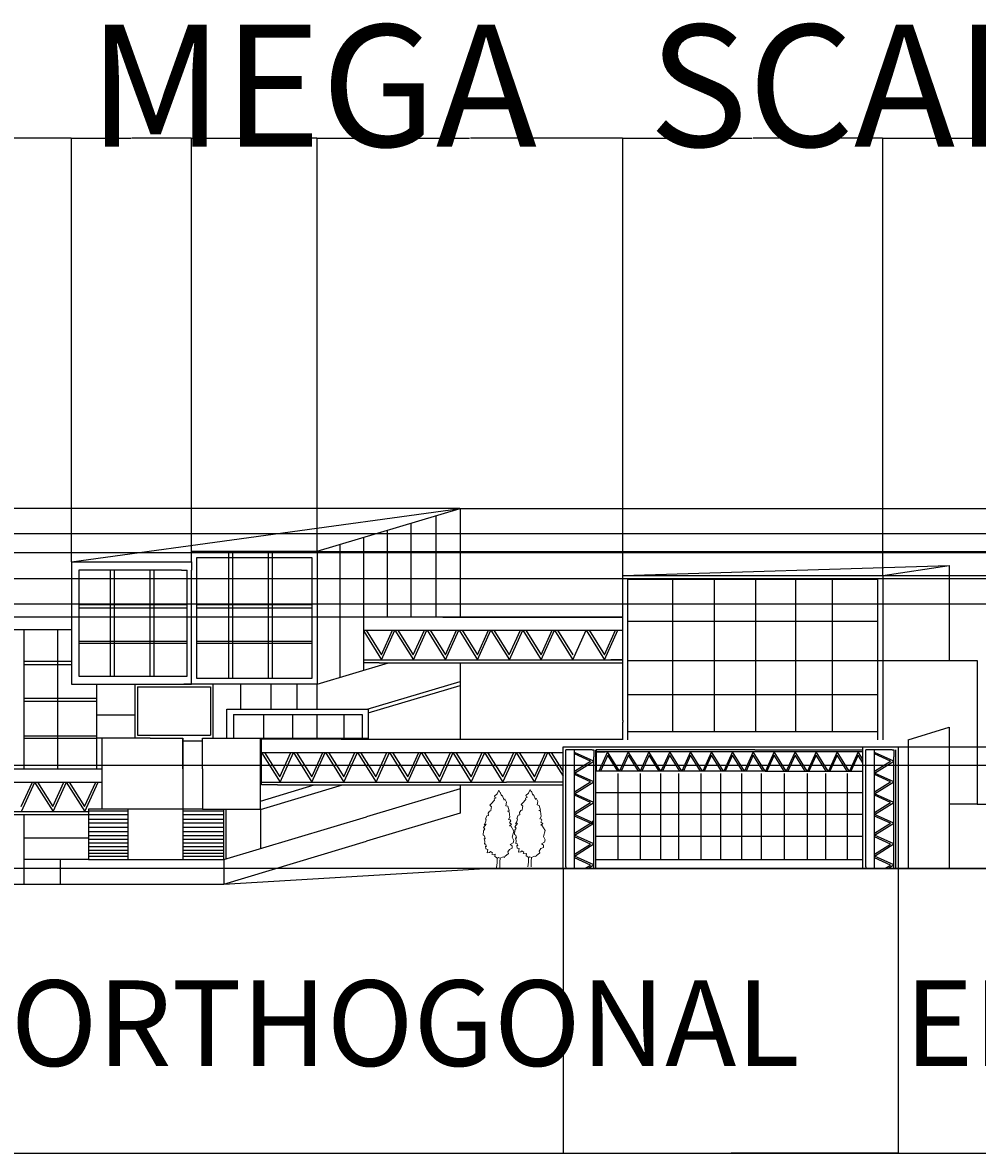
# Model space of a CAD drawing. Units: inches. Extents: x -2248 to 2617, y -128 to 922.
# Tile 2 of 7: x -1531 to -646, y -128 to 922. Entities that reach past the tile are written whole.
import ezdxf

# ---------------------------------------------------------------- set-up
doc = ezdxf.new("R2010")
doc.units = ezdxf.units.IN
doc.header["$MEASUREMENT"] = 0
for name, color, linetype, lineweight in [('A-ANNO-DIMS', 2, 'Continuous', 18), ('A-ANNO-TEXT', 7, 'Continuous', 25), ('A-ELEV', 7, 'Continuous', 25), ('L-PLNT', 3, 'Continuous', 18)]:
    doc.layers.add(name, color=color, linetype=linetype, lineweight=lineweight)
doc.styles.get("Standard").update_dxf_attribs({"font": 'arial.ttf'})
doc.dimstyles.get("Standard").update_dxf_attribs({"dimtxt": 0.18, "dimasz": 0.18, "dimexe": 0.18, "dimexo": 0.0625, "dimgap": 0.09, "dimtad": 0, "dimtih": 1, "dimtoh": 1, "dimdec": 4, "dimzin": 0, "dimdsep": 46, "dimtxsty": 'Standard', "dimcen": 0.09, "dimadec": 0, "dimazin": 0, "dimtfac": 1, "dimtdec": 4, "dimtofl": 0, "dimtmove": 0, "dimatfit": 3, "dimfxl": 1, "dimtolj": 1, "dimtzin": 0, "dimarcsym": 0})

# ---------------------------------------------------------------- blocks, each defined once
blk = doc.blocks.new('*U3')
blk.add_lwpolyline([(-2.754, 191.699), (-6.78, 182.851), (-13.682, 176.953), (-11.956, 173.266), (-9.656, 172.529), (-14.257, 170.317), (-13.682, 167.368), (-21.733, 157.783), (-25.184, 154.834), (-21.158, 150.41), (-21.733, 147.461), (-22.884, 140.825), (-26.334, 140.087), (-29.21, 134.926), (-28.635, 129.028), (-32.661, 128.291), (-36.111, 120.18), (-34.386, 118.706), (-35.536, 111.333), (-38.987, 106.171), (-34.386, 107.646), (-40.712, 98.798), (-37.261, 95.849), (-40.712, 90.688), (-41.287, 80.366), (-38.412, 78.154), (-36.686, 70.781), (-39.562, 71.518), (-37.261, 64.145), (-38.412, 57.509), (-36.111, 58.247), (-33.236, 52.348), (-35.536, 53.086), (-34.961, 46.45), (-30.36, 44.975), (-31.51, 36.128), (-26.334, 36.865), (-23.459, 39.814), (-18.283, 36.128), (-20.008, 33.178), (-14.832, 31.704), (-11.956, 33.178), (-12.531, 27.28), (-6.205, 22.856), (-3.905, 24.331), (0.121, 22.856), (8.173, 26.543), (11.624, 25.068), (12.199, 27.28), (21.4, 34.653), (19.675, 39.077), (23.701, 44.975), (30.027, 47.924), (30.602, 53.823), (25.426, 56.772), (32.903, 61.196), (34.053, 67.094), (30.602, 75.205), (34.628, 89.951), (26.576, 103.222), (23.701, 103.222), (28.302, 107.646), (23.701, 110.595), (26.576, 115.756), (25.426, 117.968), (20.825, 118.706), (24.276, 124.604), (22.551, 137.876), (19.1, 139.35), (22.551, 140.825), (19.675, 151.884), (14.499, 153.359), (16.224, 162.207), (12.199, 170.317), (10.473, 167.368), (5.872, 179.165), (4.147, 177.69), (0.696, 187.275), (-0.454, 185.8)], close=True)
for points in [[(-6.813, 23.669), (-6.813, 11.669), (-8.627, 0)], [(0.387, 23.669), (-0.576, 13.271), (-0.576, 3.686), (0, 0)]]:
    blk.add_lwpolyline(points)
blk = doc.blocks.new('*D19')
at = {"layer": 'A-ANNO-DIMS', "color": 0, "lineweight": -2, "transparency": 16777216}
for p, q in [((-1125.5, 470.6), (-2247.7, 470.6)), ((-2247.5, 470.4), (-2247.5, 438.4)), ((-2247.5, 406), (-2247.5, 438)), ((-1769.5, 405.8), (-2247.7, 405.8))]:
    blk.add_line(p, q, dxfattribs=at)
at = {"layer": 'A-ANNO-DIMS', "color": 0, "transparency": 16777216}
for points in [[(-2247.5, 470.4), (-2247.5, 470.4), (-2247.5, 470.6)], [(-2247.5, 406), (-2247.5, 406), (-2247.5, 405.8)]]:
    blk.add_solid(points, dxfattribs=at)
at = {"layer": 'Defpoints', "color": 0, "transparency": 16777216}
for p in [(-1125.4, 470.6), (-2247.5, 405.8), (-1769.4, 405.8)]:
    blk.add_point(p, dxfattribs=at)
at = {"layer": 'A-ANNO-DIMS', "color": 0, "transparency": 16777216, "insert": (-2247.5, 438.2), "char_height": 0.18, "attachment_point": 5}
blk.add_mtext('\\A1;64.83', dxfattribs=at)
blk = doc.blocks.new('*D20')
at = {"layer": 'A-ANNO-DIMS', "color": 0, "lineweight": -2, "transparency": 16777216}
for p, q in [((-1595.3, 429.9), (2616.5, 429.9)), ((2616.3, 429.7), (2616.3, 417.9)), ((2616.3, 405.8), (2616.3, 417.5)), ((-1653.9, 405.6), (2616.5, 405.6))]:
    blk.add_line(p, q, dxfattribs=at)
at = {"layer": 'A-ANNO-DIMS', "color": 0, "transparency": 16777216}
for points in [[(2616.2, 429.7), (2616.3, 429.7), (2616.3, 429.9)], [(2616.2, 405.8), (2616.3, 405.8), (2616.3, 405.6)]]:
    blk.add_solid(points, dxfattribs=at)
at = {"layer": 'Defpoints', "color": 0, "transparency": 16777216}
for p in [(-1595.4, 429.9), (-1654, 405.6), (2616.3, 405.6)]:
    blk.add_point(p, dxfattribs=at)
at = {"layer": 'A-ANNO-DIMS', "color": 0, "transparency": 16777216, "insert": (2616.3, 417.7), "char_height": 0.18, "attachment_point": 5}
blk.add_mtext('\\A1;24.3', dxfattribs=at)
blk = doc.blocks.new('*D21')
at = {"layer": 'A-ANNO-DIMS', "color": 0, "lineweight": -2, "transparency": 16777216}
for p, q in [((-1125.3, 470.6), (2616.5, 470.6)), ((2616.3, 470.4), (2616.3, 451)), ((2616.3, 431.1), (2616.3, 450.6)), ((-1257.9, 430.9), (2616.5, 430.9))]:
    blk.add_line(p, q, dxfattribs=at)
at = {"layer": 'A-ANNO-DIMS', "color": 0, "transparency": 16777216}
for points in [[(2616.2, 470.4), (2616.3, 470.4), (2616.3, 470.6)], [(2616.2, 431.1), (2616.3, 431.1), (2616.3, 430.9)]]:
    blk.add_solid(points, dxfattribs=at)
at = {"layer": 'Defpoints', "color": 0, "transparency": 16777216}
for p in [(-1125.4, 470.6), (-1258, 430.9), (2616.3, 430.9)]:
    blk.add_point(p, dxfattribs=at)
at = {"layer": 'A-ANNO-DIMS', "color": 0, "transparency": 16777216, "insert": (2616.3, 450.8), "char_height": 0.18, "attachment_point": 5}
blk.add_mtext('\\A1;39.705', dxfattribs=at)
blk = doc.blocks.new('*D22')
at = {"layer": 'A-ANNO-DIMS', "color": 0, "lineweight": -2, "transparency": 16777216}
for p, q in [((-733.3, 408.4), (2616.5, 408.4)), ((2616.3, 408.2), (2616.3, 329.1)), ((2616.3, 249.6), (2616.3, 328.7)), ((-719.1, 249.4), (2616.5, 249.4))]:
    blk.add_line(p, q, dxfattribs=at)
at = {"layer": 'A-ANNO-DIMS', "color": 0, "transparency": 16777216}
for points in [[(2616.2, 408.2), (2616.3, 408.2), (2616.3, 408.4)], [(2616.2, 249.6), (2616.3, 249.6), (2616.3, 249.4)]]:
    blk.add_solid(points, dxfattribs=at)
at = {"layer": 'Defpoints', "color": 0, "transparency": 16777216}
for p in [(-733.4, 408.4), (-719.2, 249.4), (2616.3, 249.4)]:
    blk.add_point(p, dxfattribs=at)
at = {"layer": 'A-ANNO-DIMS', "color": 0, "transparency": 16777216, "insert": (2616.3, 328.9), "char_height": 0.18, "attachment_point": 5}
blk.add_mtext('\\A1;159.02', dxfattribs=at)
blk = doc.blocks.new('*D23')
at = {"layer": 'A-ANNO-DIMS', "color": 0, "lineweight": -2, "transparency": 16777216}
for p, q in [((-719.1, 249.4), (2616.5, 249.4)), ((2616.3, 249.2), (2616.3, 193.1)), ((2616.3, 136.6), (2616.3, 192.7)), ((-719.1, 136.5), (2616.5, 136.5))]:
    blk.add_line(p, q, dxfattribs=at)
at = {"layer": 'A-ANNO-DIMS', "color": 0, "transparency": 16777216}
for points in [[(2616.2, 249.2), (2616.3, 249.2), (2616.3, 249.4)], [(2616.2, 136.6), (2616.3, 136.6), (2616.3, 136.5)]]:
    blk.add_solid(points, dxfattribs=at)
at = {"layer": 'Defpoints', "color": 0, "transparency": 16777216}
for p in [(-719.2, 249.4), (-719.2, 136.5), (2616.3, 136.5)]:
    blk.add_point(p, dxfattribs=at)
at = {"layer": 'A-ANNO-DIMS', "color": 0, "transparency": 16777216, "insert": (2616.3, 192.9), "char_height": 0.18, "attachment_point": 5}
blk.add_mtext('\\A1;112.94', dxfattribs=at)
blk = doc.blocks.new('*D29')
at = {"layer": 'A-ANNO-DIMS', "color": 0, "lineweight": -2, "transparency": 16777216}
for p, q in [((358.9, 382), (-2247.7, 382)), ((-2247.5, 381.8), (-2247.5, 259.4)), ((-2247.5, 136.6), (-2247.5, 259)), ((392.6, 136.5), (-2247.7, 136.5))]:
    blk.add_line(p, q, dxfattribs=at)
at = {"layer": 'A-ANNO-DIMS', "color": 0, "transparency": 16777216}
for points in [[(-2247.5, 381.8), (-2247.5, 381.8), (-2247.5, 382)], [(-2247.5, 136.6), (-2247.5, 136.6), (-2247.5, 136.5)]]:
    blk.add_solid(points, dxfattribs=at)
at = {"layer": 'Defpoints', "color": 0, "transparency": 16777216}
for p in [(359, 382), (-2247.5, 136.5), (392.7, 136.5)]:
    blk.add_point(p, dxfattribs=at)
at = {"layer": 'A-ANNO-DIMS', "color": 0, "transparency": 16777216, "insert": (-2247.5, 259.2), "char_height": 0.18, "attachment_point": 5}
blk.add_mtext('\\A1;245.5', dxfattribs=at)
blk = doc.blocks.new('*D30')
at = {"layer": 'A-ANNO-DIMS', "color": 0, "lineweight": -2, "transparency": 16777216}
for p, q in [((201.8, 232.1), (-2247.7, 232.1)), ((-2247.5, 231.9), (-2247.5, 184.4)), ((-2247.5, 136.6), (-2247.5, 184.1)), ((210.7, 136.5), (-2247.7, 136.5))]:
    blk.add_line(p, q, dxfattribs=at)
at = {"layer": 'A-ANNO-DIMS', "color": 0, "transparency": 16777216}
for points in [[(-2247.5, 231.9), (-2247.5, 231.9), (-2247.5, 232.1)], [(-2247.5, 136.6), (-2247.5, 136.6), (-2247.5, 136.5)]]:
    blk.add_solid(points, dxfattribs=at)
at = {"layer": 'Defpoints', "color": 0, "transparency": 16777216}
for p in [(201.8, 232.1), (-2247.5, 136.5), (210.8, 136.5)]:
    blk.add_point(p, dxfattribs=at)
at = {"layer": 'A-ANNO-DIMS', "color": 0, "transparency": 16777216, "insert": (-2247.5, 184.3), "char_height": 0.18, "attachment_point": 5}
blk.add_mtext('\\A1;95.6', dxfattribs=at)
blk = doc.blocks.new('*D31')
at = {"layer": 'A-ANNO-DIMS', "color": 0, "lineweight": -2, "transparency": 16777216}
for p, q in [((934.8, 447.2), (-2247.7, 447.2)), ((-2247.5, 447), (-2247.5, 292)), ((-2247.5, 136.6), (-2247.5, 291.6)), ((820, 136.5), (-2247.7, 136.5))]:
    blk.add_line(p, q, dxfattribs=at)
at = {"layer": 'A-ANNO-DIMS', "color": 0, "transparency": 16777216}
for points in [[(-2247.5, 447), (-2247.5, 447), (-2247.5, 447.2)], [(-2247.5, 136.6), (-2247.5, 136.6), (-2247.5, 136.5)]]:
    blk.add_solid(points, dxfattribs=at)
at = {"layer": 'Defpoints', "color": 0, "transparency": 16777216}
for p in [(934.9, 447.2), (-2247.5, 136.5), (820.1, 136.5)]:
    blk.add_point(p, dxfattribs=at)
at = {"layer": 'A-ANNO-DIMS', "color": 0, "transparency": 16777216, "insert": (-2247.5, 291.8), "char_height": 0.18, "attachment_point": 5}
blk.add_mtext('\\A1;310.7', dxfattribs=at)
blk = doc.blocks.new('*D32')
at = {"layer": 'A-ANNO-DIMS', "color": 0, "lineweight": -2, "transparency": 16777216}
for p, q in [((-975.3, 369.9), (-2247.7, 369.9)), ((-2247.5, 369.8), (-2247.5, 253.4)), ((-2247.5, 136.6), (-2247.5, 253)), ((-1029.9, 136.5), (-2247.7, 136.5))]:
    blk.add_line(p, q, dxfattribs=at)
at = {"layer": 'A-ANNO-DIMS', "color": 0, "transparency": 16777216}
for points in [[(-2247.5, 369.8), (-2247.5, 369.8), (-2247.5, 369.9)], [(-2247.5, 136.6), (-2247.5, 136.6), (-2247.5, 136.5)]]:
    blk.add_solid(points, dxfattribs=at)
at = {"layer": 'Defpoints', "color": 0, "transparency": 16777216}
for p in [(-975.2, 369.9), (-2247.5, 136.5), (-1029.8, 136.5)]:
    blk.add_point(p, dxfattribs=at)
at = {"layer": 'A-ANNO-DIMS', "color": 0, "transparency": 16777216, "insert": (-2247.5, 253.2), "char_height": 0.18, "attachment_point": 5}
blk.add_mtext('\\A1;233.5', dxfattribs=at)
blk = doc.blocks.new('*D33')
at = {"layer": 'A-ANNO-DIMS', "color": 0, "lineweight": -2, "transparency": 16777216}
for p, q in [((2393, 136.4), (2393, -127.9)), ((-2024.3, 122), (-2024.3, -127.9)), ((-2024.1, -127.7), (184, -127.7)), ((2392.8, -127.7), (184.7, -127.7))]:
    blk.add_line(p, q, dxfattribs=at)
at = {"layer": 'A-ANNO-DIMS', "color": 0, "transparency": 16777216}
for points in [[(-2024.1, -127.6), (-2024.1, -127.7), (-2024.3, -127.7)], [(2392.8, -127.6), (2392.8, -127.7), (2393, -127.7)]]:
    blk.add_solid(points, dxfattribs=at)
at = {"layer": 'Defpoints', "color": 0, "transparency": 16777216}
for p in [(2393, 136.5), (-2024.3, 122.1), (2393, -127.7)]:
    blk.add_point(p, dxfattribs=at)
at = {"layer": 'A-ANNO-DIMS', "color": 0, "transparency": 16777216, "insert": (184.4, -127.7), "char_height": 0.18, "attachment_point": 5}
blk.add_mtext('\\A1;4417', dxfattribs=at)
blk = doc.blocks.new('*D36')
at = {"layer": 'A-ANNO-DIMS', "color": 0, "lineweight": -2, "transparency": 16777216}
for p, q in [((-1654, 405.6), (-1654, 814.7)), ((-1653.8, 814.5), (-1570.3, 814.5)), ((-1486, 814.5), (-1569.4, 814.5)), ((-1485.8, 421.2), (-1485.8, 814.7))]:
    blk.add_line(p, q, dxfattribs=at)
at = {"layer": 'A-ANNO-DIMS', "color": 0, "transparency": 16777216}
for points in [[(-1653.8, 814.5), (-1653.8, 814.5), (-1654, 814.5)], [(-1486, 814.5), (-1486, 814.5), (-1485.8, 814.5)]]:
    blk.add_solid(points, dxfattribs=at)
at = {"layer": 'Defpoints', "color": 0, "transparency": 16777216}
for p in [(-1485.8, 814.5), (-1485.8, 421.2), (-1654, 405.6)]:
    blk.add_point(p, dxfattribs=at)
at = {"layer": 'A-ANNO-DIMS', "color": 0, "transparency": 16777216, "insert": (-1569.9, 814.5), "char_height": 0.18, "attachment_point": 5}
blk.add_mtext('\\A1;168.15', dxfattribs=at)
blk = doc.blocks.new('*D37')
at = {"layer": 'A-ANNO-DIMS', "color": 0, "lineweight": -2, "transparency": 16777216}
for p, q in [((-1485.8, 421.2), (-1485.8, 814.7)), ((-1485.6, 814.5), (-1430.6, 814.5)), ((-1374.8, 814.5), (-1429.8, 814.5)), ((-1374.6, 421.2), (-1374.6, 814.7))]:
    blk.add_line(p, q, dxfattribs=at)
at = {"layer": 'A-ANNO-DIMS', "color": 0, "transparency": 16777216}
for points in [[(-1485.6, 814.5), (-1485.6, 814.5), (-1485.8, 814.5)], [(-1374.8, 814.5), (-1374.8, 814.5), (-1374.6, 814.5)]]:
    blk.add_solid(points, dxfattribs=at)
at = {"layer": 'Defpoints', "color": 0, "transparency": 16777216}
for p in [(-1374.6, 814.5), (-1485.8, 421.2), (-1374.6, 421.2)]:
    blk.add_point(p, dxfattribs=at)
at = {"layer": 'A-ANNO-DIMS', "color": 0, "transparency": 16777216, "insert": (-1430.2, 814.5), "char_height": 0.18, "attachment_point": 5}
blk.add_mtext('\\A1;111.2', dxfattribs=at)
blk = doc.blocks.new('*D38')
at = {"layer": 'A-ANNO-DIMS', "color": 0, "lineweight": -2, "transparency": 16777216}
for p, q in [((-1374.6, 431), (-1374.6, 814.7)), ((-1374.4, 814.5), (-1316.7, 814.5)), ((-1258.1, 814.5), (-1315.8, 814.5)), ((-1258, 431), (-1258, 814.7))]:
    blk.add_line(p, q, dxfattribs=at)
at = {"layer": 'A-ANNO-DIMS', "color": 0, "transparency": 16777216}
for points in [[(-1374.4, 814.5), (-1374.4, 814.5), (-1374.6, 814.5)], [(-1258.1, 814.5), (-1258.1, 814.5), (-1258, 814.5)]]:
    blk.add_solid(points, dxfattribs=at)
at = {"layer": 'Defpoints', "color": 0, "transparency": 16777216}
for p in [(-1258, 814.5), (-1374.6, 430.9), (-1258, 430.9)]:
    blk.add_point(p, dxfattribs=at)
at = {"layer": 'A-ANNO-DIMS', "color": 0, "transparency": 16777216, "insert": (-1316.3, 814.5), "char_height": 0.18, "attachment_point": 5}
blk.add_mtext('\\A1;116.66', dxfattribs=at)
blk = doc.blocks.new('*D39')
at = {"layer": 'A-ANNO-DIMS', "color": 0, "lineweight": -2, "transparency": 16777216}
for p, q in [((-1258, 431), (-1258, 814.7)), ((-1257.8, 814.5), (-1116.7, 814.5)), ((-974.6, 814.5), (-1115.7, 814.5)), ((-974.4, 408.5), (-974.4, 814.7))]:
    blk.add_line(p, q, dxfattribs=at)
at = {"layer": 'A-ANNO-DIMS', "color": 0, "transparency": 16777216}
for points in [[(-1257.8, 814.5), (-1257.8, 814.5), (-1258, 814.5)], [(-974.6, 814.5), (-974.6, 814.5), (-974.4, 814.5)]]:
    blk.add_solid(points, dxfattribs=at)
at = {"layer": 'Defpoints', "color": 0, "transparency": 16777216}
for p in [(-974.4, 814.5), (-1258, 430.9), (-974.4, 408.4)]:
    blk.add_point(p, dxfattribs=at)
at = {"layer": 'A-ANNO-DIMS', "color": 0, "transparency": 16777216, "insert": (-1116.2, 814.5), "char_height": 0.18, "attachment_point": 5}
blk.add_mtext('\\A1;283.54', dxfattribs=at)
blk = doc.blocks.new('*D40')
at = {"layer": 'A-ANNO-DIMS', "color": 0, "lineweight": -2, "transparency": 16777216}
for p, q in [((-974.4, 408.5), (-974.4, 814.7)), ((-974.2, 814.5), (-854.4, 814.5)), ((-733.6, 814.5), (-853.4, 814.5)), ((-733.4, 408.5), (-733.4, 814.7))]:
    blk.add_line(p, q, dxfattribs=at)
at = {"layer": 'A-ANNO-DIMS', "color": 0, "transparency": 16777216}
for points in [[(-974.2, 814.5), (-974.2, 814.5), (-974.4, 814.5)], [(-733.6, 814.5), (-733.6, 814.5), (-733.4, 814.5)]]:
    blk.add_solid(points, dxfattribs=at)
at = {"layer": 'Defpoints', "color": 0, "transparency": 16777216}
for p in [(-733.4, 814.5), (-974.4, 408.4), (-733.4, 408.4)]:
    blk.add_point(p, dxfattribs=at)
at = {"layer": 'A-ANNO-DIMS', "color": 0, "transparency": 16777216, "insert": (-853.9, 814.5), "char_height": 0.18, "attachment_point": 5}
blk.add_mtext('\\A1;241.04', dxfattribs=at)
blk = doc.blocks.new('*D41')
at = {"layer": 'A-ANNO-DIMS', "color": 0, "lineweight": -2, "transparency": 16777216}
for p, q in [((-733.4, 408.5), (-733.4, 814.7)), ((-733.2, 814.5), (-649, 814.5)), ((-564.1, 814.5), (-648.2, 814.5)), ((-563.9, 327), (-563.9, 814.7))]:
    blk.add_line(p, q, dxfattribs=at)
at = {"layer": 'A-ANNO-DIMS', "color": 0, "transparency": 16777216}
for points in [[(-733.2, 814.5), (-733.2, 814.5), (-733.4, 814.5)], [(-564.1, 814.5), (-564.1, 814.5), (-563.9, 814.5)]]:
    blk.add_solid(points, dxfattribs=at)
at = {"layer": 'Defpoints', "color": 0, "transparency": 16777216}
for p in [(-563.9, 814.5), (-733.4, 408.4), (-563.9, 326.9)]:
    blk.add_point(p, dxfattribs=at)
at = {"layer": 'A-ANNO-DIMS', "color": 0, "transparency": 16777216, "insert": (-648.6, 814.5), "char_height": 0.18, "attachment_point": 5}
blk.add_mtext('\\A1;169.5', dxfattribs=at)
blk = doc.blocks.new('*D55')
at = {"layer": 'A-ANNO-DIMS', "color": 0, "lineweight": -2, "transparency": 16777216}
for p, q in [((-1029.8, 136.4), (-1029.8, -127.9)), ((-719.2, 136.4), (-719.2, -127.9)), ((-1029.6, -127.7), (-874.9, -127.7)), ((-719.4, -127.7), (-874.1, -127.7))]:
    blk.add_line(p, q, dxfattribs=at)
at = {"layer": 'A-ANNO-DIMS', "color": 0, "transparency": 16777216}
for points in [[(-1029.6, -127.6), (-1029.6, -127.7), (-1029.8, -127.7)], [(-719.4, -127.6), (-719.4, -127.7), (-719.2, -127.7)]]:
    blk.add_solid(points, dxfattribs=at)
at = {"layer": 'Defpoints', "color": 0, "transparency": 16777216}
for p in [(-1029.8, 136.5), (-719.2, 136.5), (-719.2, -127.7)]:
    blk.add_point(p, dxfattribs=at)
at = {"layer": 'A-ANNO-DIMS', "color": 0, "transparency": 16777216, "insert": (-874.5, -127.7), "char_height": 0.18, "attachment_point": 5}
blk.add_mtext('\\A1;310.6', dxfattribs=at)

msp = doc.modelspace()

# ---------------------------------------------------------------- linework, layer by layer
at = {"layer": 'A-ELEV'}
for p, q in [((-1485.8077, 421.1696), (-1125.4072, 470.6286)), ((-1257.9572, 430.9238), (-1125.4072, 470.6286)), ((-1147.628, 369.9469), (-1147.628, 463.9724)), ((-1125.4072, 470.6286), (-1125.4072, 369.9469)), ((-1170.7914, 369.9469), (-1170.7914, 457.0339)), ((-1214.6825, 320.7275), (-1214.6825, 443.8866)), ((-1192.7139, 369.9469), (-1192.7139, 450.4672)), ((-1374.6151, 421.1696), (-1374.6151, 430.9238)), ((-1374.6151, 430.9238), (-1257.9572, 430.9238)), ((-1339.8325, 312.9553), (-1339.8325, 430.9238)), ((-1336.0257, 312.9553), (-1336.0257, 430.9238)), ((-1303.0376, 312.9553), (-1303.0376, 430.9238)), ((-1299.2308, 312.9553), (-1299.2308, 430.9238)), ((-1257.9572, 430.9238), (-1257.9572, 307.4874)), ((-1236.5303, 314.1831), (-1236.5303, 437.3422)), ((-1485.8077, 421.1696), (-1485.8077, 307.4874)), ((-1485.8077, 421.1696), (-1381.4843, 421.1696)), ((-1381.4843, 421.1696), (-1374.6151, 421.1696)), ((-1374.6151, 421.1696), (-1374.6151, 413.422)), ((-1369.6504, 425.3485), (-1262.7839, 425.3485)), ((-1369.6504, 312.9553), (-1369.6504, 425.3485)), ((-1262.7839, 425.3485), (-1262.7839, 312.9553)), ((-1383.6311, 413.422), (-1478.9778, 413.422)), ((-1478.9778, 413.422), (-1478.9778, 315.1979)), ((-1449.7435, 315.1979), (-1449.7435, 413.422)), ((-1445.9367, 315.1979), (-1445.9367, 413.422)), ((-1412.9486, 315.1979), (-1412.9486, 413.422)), ((-1409.1418, 315.1979), (-1409.1418, 413.422)), ((-1383.6311, 413.422), (-1378.4219, 413.422)), ((-1378.4219, 315.1979), (-1378.4219, 413.422)), ((-1374.6151, 315.1979), (-1374.6151, 413.422)), ((-974.4198, 408.4102), (-671.7685, 417.6576)), ((-733.3752, 408.4102), (-671.7685, 417.6576)), ((-671.7685, 417.6576), (-671.7685, 329.7298)), ((-974.4198, 273.9094), (-974.4198, 408.4102)), ((-974.4198, 408.4102), (-733.3752, 408.4102)), ((-969.8646, 256.0775), (-969.8646, 405.203)), ((-969.8646, 405.203), (-738.371, 405.203)), ((-928.1701, 263.754), (-928.1701, 405.203)), ((-889.2644, 263.754), (-889.2644, 405.203)), ((-851.0598, 263.754), (-851.0598, 405.203)), ((-813.9067, 263.754), (-813.9067, 405.203)), ((-779.9081, 263.754), (-779.9081, 405.203)), ((-738.371, 405.203), (-738.371, 256.0775)), ((-733.3752, 408.4102), (-733.3752, 256.0775)), ((-1478.9778, 381.455), (-1378.4219, 381.455)), ((-1478.9778, 378.5661), (-1378.4219, 378.5661)), ((-1369.6504, 381.455), (-1262.7839, 381.455)), ((-1369.6504, 378.5661), (-1262.7839, 378.5661)), ((-1141.4884, 369.9469), (-1214.6825, 369.9469)), ((-1141.4884, 369.9469), (-975.2258, 369.9469)), ((-1595.3791, 358.31), (-1530.0359, 358.31)), ((-1530.0359, 358.31), (-1530.0359, 229.0275)), ((-1530.0359, 358.31), (-1485.8077, 358.31)), ((-1498.4948, 229.0275), (-1498.4948, 358.31)), ((-1214.6825, 357.7454), (-975.2258, 357.7454)), ((-1212.5193, 357.7367), (-1198.313, 334.9981)), ((-1198.313, 334.9981), (-1188.0363, 357.7454)), ((-1198.1833, 330.2906), (-1185.7808, 357.7433)), ((-1185.8244, 357.7454), (-1168.6715, 330.2906)), ((-1183.0075, 357.7367), (-1168.8011, 334.9981)), ((-1168.8011, 334.9981), (-1158.5244, 357.7454)), ((-1168.6715, 330.2906), (-1156.269, 357.7433)), ((-1156.0059, 357.7454), (-1138.853, 330.2906)), ((-1153.189, 357.7367), (-1138.9827, 334.9981)), ((-1138.9827, 334.9981), (-1128.7059, 357.7454)), ((-1138.853, 330.2906), (-1126.4505, 357.7433)), ((-1126.2751, 357.7454), (-1109.1222, 330.2906)), ((-1123.4582, 357.7367), (-1109.2519, 334.9981)), ((-1109.2519, 334.9981), (-1098.9752, 357.7454)), ((-1109.1222, 330.2906), (-1096.7197, 357.7433)), ((-1096.7476, 357.7454), (-1079.5947, 330.2906)), ((-1093.9307, 357.7367), (-1079.7243, 334.9981)), ((-1079.7243, 334.9981), (-1069.4476, 357.7454)), ((-1079.5947, 330.2906), (-1067.1922, 357.7433)), ((-1067.22, 357.7454), (-1050.0671, 330.2906)), ((-1064.4031, 357.7367), (-1050.1968, 334.9981)), ((-1050.1968, 334.9981), (-1039.9201, 357.7454)), ((-1050.0671, 330.2906), (-1037.6646, 357.7433)), ((-1037.918, 357.7454), (-1020.765, 330.2906)), ((-1035.101, 357.7367), (-1020.8947, 334.9981)), ((-1020.765, 330.2906), (-1008.3625, 357.7433)), ((-1008.5359, 357.7454), (-991.3829, 330.2906)), ((-1005.7189, 357.7367), (-991.5126, 334.9981)), ((-991.5126, 334.9981), (-981.2359, 357.7454)), ((-991.3829, 330.2906), (-978.9804, 357.7433)), ((-969.8646, 365.9872), (-738.371, 365.9872)), ((-1478.9778, 347.6299), (-1378.4219, 347.6299)), ((-1369.6504, 347.6299), (-1262.7839, 347.6299)), ((-1214.6825, 356.6991), (-1198.1833, 330.2906)), ((-1478.9778, 345.6601), (-1378.4219, 345.6601)), ((-1369.6504, 345.6601), (-1262.7839, 345.6601)), ((-1530.0359, 328.9999), (-1485.8077, 328.9999)), ((-1530.0359, 325.9078), (-1485.8077, 325.9078)), ((-1257.9572, 307.7647), (-1191.8127, 327.578)), ((-1214.6825, 330.2635), (-974.4198, 330.2635)), ((-1200.437, 327.578), (-1214.6825, 327.578)), ((-1200.437, 327.578), (-974.4198, 327.578)), ((-1125.4072, 327.578), (-1125.4072, 256.4375)), ((-987.9902, 327.578), (-975.2258, 327.578)), ((-975.2258, 330.2635), (-985.4566, 330.2635)), ((-969.8646, 329.7298), (-738.371, 329.7298)), ((-738.371, 329.7298), (-645.8648, 329.7298)), ((-645.8648, 329.7298), (-645.8648, 196.2696)), ((-1478.9778, 315.1979), (-1381.4843, 315.1979)), ((-1381.4843, 315.1979), (-1378.4219, 315.1979)), ((-1374.6151, 307.4874), (-1374.6151, 315.1979)), ((-1485.8077, 307.4874), (-1381.4843, 307.4874)), ((-1462.7609, 307.4874), (-1462.7609, 229.0275)), ((-1426.9499, 307.4874), (-1426.9499, 257.552)), ((-1424.4443, 305.1388), (-1424.4443, 260.2412)), ((-1424.4443, 305.1388), (-1356.8422, 305.1388)), ((-1381.4843, 307.4874), (-1374.6151, 307.4874)), ((-1257.9572, 307.4874), (-1381.4843, 307.4874)), ((-1262.7839, 312.9553), (-1369.6504, 312.9553)), ((-1356.8422, 305.1388), (-1356.8422, 260.2412)), ((-1354.5526, 257.552), (-1354.5526, 307.4874)), ((-1328.7904, 284.3577), (-1328.7904, 307.4874)), ((-1300.4636, 284.3577), (-1300.4636, 307.4874)), ((-1276.6333, 284.3577), (-1276.6333, 307.4874)), ((-1257.9572, 284.3577), (-1257.9572, 307.4874)), ((-1211.7192, 284.3577), (-1125.4072, 310.2121)), ((-1210.5891, 280.9745), (-1125.4072, 306.4903)), ((-1530.0359, 294.6973), (-1462.7609, 294.6973)), ((-974.4198, 273.9094), (-974.4198, 298.3514)), ((-969.8646, 298.1516), (-738.371, 298.1516)), ((-1530.0359, 291.9114), (-1462.7609, 291.9114)), ((-1341.6517, 257.552), (-1341.6517, 284.3577)), ((-1341.6517, 284.3577), (-1210.5891, 284.3577)), ((-1210.5891, 284.3577), (-1210.5891, 256.4375)), ((-1462.7609, 279.1363), (-1426.9499, 279.1363)), ((-1335.6667, 279.3427), (-1216.2013, 279.3427)), ((-1335.6667, 279.3427), (-1335.6667, 257.552)), ((-1307.2842, 257.552), (-1307.2842, 279.3427)), ((-1280.4676, 257.552), (-1280.4676, 279.3427)), ((-1257.9927, 257.552), (-1257.9927, 279.3427)), ((-1232.9967, 257.552), (-1232.9967, 279.3427)), ((-1216.2013, 279.3427), (-1216.2013, 257.552)), ((-974.4198, 273.9094), (-974.4198, 272.4308)), ((-974.4198, 256.0775), (-974.4198, 272.4308)), ((-969.8646, 263.754), (-738.371, 263.754)), ((-709.8168, 256.0775), (-671.7685, 267.5832)), ((-671.7685, 267.5832), (-671.7685, 196.2696)), ((-1530.0359, 259.7188), (-1462.7609, 259.7188)), ((-1530.0359, 257.552), (-1462.7609, 257.552)), ((-1412.9486, 257.552), (-1462.7609, 257.552)), ((-1457.3701, 229.0275), (-1457.3701, 257.552)), ((-1424.4443, 260.2412), (-1356.8422, 260.2412)), ((-1412.9486, 257.552), (-1382.6193, 257.552)), ((-1382.6193, 229.0275), (-1382.6193, 257.552)), ((-1382.6193, 257.552), (-1382.6193, 191.6077)), ((-1382.6193, 255.0357), (-1364.4124, 255.0357)), ((-1364.4124, 229.0275), (-1364.4124, 257.552)), ((-1364.4124, 257.552), (-1257.9572, 257.552)), ((-1310.5836, 229.0275), (-1310.5836, 257.552)), ((-1235.7073, 256.4375), (-1310.5836, 256.4375)), ((-1309.5551, 216.754), (-1309.5551, 256.4375)), ((-1257.9927, 257.552), (-1210.5891, 257.552)), ((-1257.9572, 257.552), (-1257.9572, 257.7708)), ((-1235.7073, 256.4375), (-974.4198, 256.4375)), ((-709.8168, 256.0775), (-709.8168, 136.4519)), ((-1309.5551, 244.236), (-1029.8099, 244.236)), ((-1309.5551, 244.236), (-1292.4022, 216.7812)), ((-1306.7382, 244.2273), (-1292.5319, 221.4887)), ((-1292.5319, 221.4887), (-1282.2552, 244.236)), ((-1292.4022, 216.7812), (-1279.9997, 244.2338)), ((-1280.0433, 244.236), (-1262.8904, 216.7812)), ((-1277.2264, 244.2273), (-1263.02, 221.4887)), ((-1263.02, 221.4887), (-1252.7433, 244.236)), ((-1262.8904, 216.7812), (-1250.4879, 244.2338)), ((-1250.2248, 244.236), (-1233.0719, 216.7812)), ((-1247.4079, 244.2273), (-1233.2016, 221.4887)), ((-1233.2016, 221.4887), (-1222.9248, 244.236)), ((-1233.0719, 216.7812), (-1220.6694, 244.2338)), ((-1220.494, 244.236), (-1203.3411, 216.7812)), ((-1217.6771, 244.2273), (-1203.4708, 221.4887)), ((-1203.4708, 221.4887), (-1193.1941, 244.236)), ((-1203.3411, 216.7812), (-1190.9386, 244.2338)), ((-1190.9665, 244.236), (-1173.8136, 216.7812)), ((-1188.1496, 244.2273), (-1173.9432, 221.4887)), ((-1173.9432, 221.4887), (-1163.6665, 244.236)), ((-1173.8136, 216.7812), (-1161.4111, 244.2338)), ((-1161.4389, 244.236), (-1144.286, 216.7812)), ((-1158.622, 244.2273), (-1144.4157, 221.4887)), ((-1144.4157, 221.4887), (-1134.139, 244.236)), ((-1144.286, 216.7812), (-1131.8835, 244.2338)), ((-1133.5882, 244.236), (-1134.2252, 244.0452)), ((-1133.5882, 244.236), (-1134.2252, 244.0452)), ((-1132.1369, 244.236), (-1114.9839, 216.7812)), ((-1129.3199, 244.2273), (-1115.1136, 221.4887)), ((-1115.1136, 221.4887), (-1104.8369, 244.236)), ((-1114.9839, 216.7812), (-1102.5814, 244.2338)), ((-1102.7548, 244.236), (-1085.6018, 216.7812)), ((-1099.9378, 244.2273), (-1085.7315, 221.4887)), ((-1085.7315, 221.4887), (-1075.4548, 244.236)), ((-1085.6018, 216.7812), (-1073.1993, 244.2338)), ((-1073.4557, 244.236), (-1056.3028, 216.7812)), ((-1070.6388, 244.2273), (-1056.4324, 221.4887)), ((-1056.4324, 221.4887), (-1046.1557, 244.236)), ((-1056.3028, 216.7812), (-1043.9003, 244.2338)), ((-1043.6169, 244.236), (-1029.8099, 222.1366)), ((-1040.8, 244.2273), (-1029.8099, 226.6366)), ((-1029.8099, 136.4519), (-1029.8099, 249.389)), ((-1029.8099, 249.389), (-719.1936, 249.389)), ((-1027.1698, 138.162), (-1027.1698, 246.762)), ((-1002.7278, 246.762), (-1027.1698, 246.762)), ((-1027.1698, 243.2408), (-1027.1698, 246.762)), ((-1019.2, 136.4519), (-1019.2, 246.762)), ((-1004.3419, 236.1238), (-1019.2, 242.8364)), ((-1001.267, 236.2085), (-1019.1986, 244.3096)), ((-1002.7278, 246.762), (-1001.2492, 246.762)), ((-1001.2492, 246.762), (-1001.2492, 240.0794)), ((-999.4951, 238.4246), (-999.4951, 246.762)), ((-990.7946, 246.7131), (-999.132, 246.7131)), ((-999.132, 246.7131), (-999.132, 243.4805)), ((-990.7946, 244.959), (-999.132, 244.959)), ((-999.132, 244.959), (-990.7946, 244.959)), ((-999.132, 243.4805), (-999.132, 227.0082)), ((-988.5785, 244.9413), (-996.6796, 227.0096)), ((-988.4938, 241.8664), (-995.2064, 227.0082)), ((-979.046, 246.7131), (-990.7946, 246.7131)), ((-751.6796, 244.959), (-990.7946, 244.959)), ((-977.3745, 227.0082), (-988.5785, 244.9413)), ((-979.2144, 227.0139), (-988.4938, 241.8664)), ((-852.0278, 246.7131), (-979.046, 246.7131)), ((-969.3866, 244.9413), (-977.4877, 227.0096)), ((-969.3019, 241.8664), (-976.0145, 227.0082)), ((-958.1826, 227.0082), (-969.3866, 244.9413)), ((-960.0225, 227.0139), (-969.3019, 241.8664)), ((-950.2469, 244.9413), (-958.348, 227.0096)), ((-950.1622, 241.8664), (-956.8748, 227.0082)), ((-939.0429, 227.0082), (-950.2469, 244.9413)), ((-940.8829, 227.0139), (-950.1622, 241.8664)), ((-947.8324, 244.9917), (-947.8503, 244.959)), ((-947.8174, 244.959), (-947.8324, 244.9917)), ((-930.96, 244.9413), (-939.0611, 227.0096)), ((-930.8753, 241.8664), (-937.5879, 227.0082)), ((-919.756, 227.0082), (-930.96, 244.9413)), ((-921.596, 227.0139), (-930.8753, 241.8664)), ((-911.6731, 244.9413), (-919.7742, 227.0096)), ((-911.5884, 241.8664), (-918.301, 227.0082)), ((-900.4691, 227.0082), (-911.6731, 244.9413)), ((-902.3091, 227.0139), (-911.5884, 241.8664)), ((-892.2534, 244.9413), (-900.3546, 227.0096)), ((-892.1687, 241.8664), (-898.8813, 227.0082)), ((-881.0494, 227.0082), (-892.2534, 244.9413)), ((-882.8894, 227.0139), (-892.1687, 241.8664)), ((-872.7765, 244.9413), (-880.8776, 227.0096)), ((-872.6918, 241.8664), (-879.4044, 227.0082)), ((-861.5725, 227.0082), (-872.7765, 244.9413)), ((-863.4125, 227.0139), (-872.6918, 241.8664)), ((-853.4998, 244.9413), (-861.601, 227.0096)), ((-853.4152, 241.8664), (-860.1277, 227.0082)), ((-842.2958, 227.0082), (-853.4998, 244.9413)), ((-844.1358, 227.0139), (-853.4152, 241.8664)), ((-852.0278, 246.5867), (-751.6796, 246.5867)), ((-834.1517, 244.9413), (-842.2528, 227.0096)), ((-834.067, 241.8664), (-840.7796, 227.0082)), ((-822.9477, 227.0082), (-834.1517, 244.9413)), ((-824.7877, 227.0139), (-834.067, 241.8664)), ((-814.7058, 244.9413), (-822.8069, 227.0096)), ((-814.6211, 241.8664), (-821.3337, 227.0082)), ((-803.5018, 227.0082), (-814.7058, 244.9413)), ((-805.3418, 227.0139), (-814.6211, 241.8664)), ((-795.2038, 244.9413), (-803.3049, 227.0096)), ((-795.1191, 241.8664), (-801.8317, 227.0082)), ((-783.9998, 227.0082), (-795.2038, 244.9413)), ((-785.8398, 227.0139), (-795.1191, 241.8664)), ((-775.6602, 244.9413), (-783.7613, 227.0096)), ((-775.5755, 241.8664), (-782.2881, 227.0082)), ((-764.4562, 227.0082), (-775.6602, 244.9413)), ((-766.2962, 227.0139), (-775.5755, 241.8664)), ((-756.2144, 244.9413), (-764.3155, 227.0096)), ((-756.1297, 241.8664), (-762.8423, 227.0082)), ((-751.6796, 237.683), (-756.2144, 244.9413)), ((-751.6796, 234.7437), (-756.1297, 241.8664)), ((-751.6796, 136.4519), (-751.6796, 249.389)), ((-749.0396, 138.162), (-749.0396, 246.762)), ((-724.5975, 246.762), (-749.0396, 246.762)), ((-749.0396, 243.2408), (-749.0396, 246.762)), ((-741.0698, 136.4519), (-741.0698, 246.762)), ((-726.2116, 236.1238), (-741.0698, 242.8364)), ((-723.1367, 236.2085), (-741.0684, 244.3096)), ((-724.5975, 246.762), (-723.119, 246.762)), ((-723.119, 246.762), (-723.119, 240.0794)), ((-721.3649, 238.4246), (-721.3649, 246.762)), ((-719.1936, 249.389), (-719.1936, 136.4519)), ((-1019.2, 225.0045), (-1001.267, 236.2085)), ((-1019.1943, 226.8444), (-1004.3419, 236.1238)), ((-1001.2492, 238.4246), (-1001.2492, 240.0794)), ((-1001.2492, 136.4519), (-1001.2492, 238.4246)), ((-999.4951, 226.676), (-999.4951, 238.4246)), ((-906.9389, 236.9224), (-906.9389, 236.9421)), ((-741.0698, 225.0045), (-723.1367, 236.2085)), ((-741.0641, 226.8444), (-726.2116, 236.1238)), ((-723.119, 238.4246), (-723.119, 240.0794)), ((-723.119, 136.4519), (-723.119, 238.4246)), ((-721.3649, 226.676), (-721.3649, 238.4246)), ((-1623.6327, 229.0275), (-1457.3701, 229.0275)), ((-1462.7609, 229.0275), (-1457.3701, 229.0275)), ((-1457.3701, 191.6077), (-1457.3701, 229.0275)), ((-1364.4124, 229.0275), (-1364.4124, 191.6077)), ((-1310.5836, 191.6077), (-1310.5836, 229.0275)), ((-1210.5891, 229.0578), (-1210.5891, 229.0275)), ((-1004.3419, 216.9319), (-1019.2, 223.6444)), ((-1001.267, 217.0165), (-1019.1986, 225.1177)), ((-999.4951, 136.4519), (-999.4951, 226.676)), ((-842.2958, 227.0082), (-999.132, 227.0082)), ((-979.2144, 224.7717), (-979.2144, 144.9711)), ((-958.4489, 224.7717), (-958.4489, 144.9711)), ((-957.2346, 227.0082), (-956.8185, 227.1329)), ((-957.2346, 227.0082), (-956.8185, 227.1329)), ((-939.6302, 224.7717), (-939.6302, 144.9711)), ((-922.7582, 224.7717), (-922.7582, 144.9711)), ((-901.9927, 224.7717), (-901.9927, 144.9711)), ((-883.8228, 224.7717), (-883.8228, 144.9711)), ((-864.3552, 224.7717), (-864.3552, 144.9711)), ((-846.1853, 224.7717), (-846.1853, 144.9711)), ((-842.2958, 227.0082), (-751.6796, 227.0082)), ((-824.7709, 224.7717), (-824.7709, 144.9711)), ((-803.3564, 224.7717), (-803.3564, 144.9711)), ((-786.4845, 224.7717), (-786.4845, 144.9711)), ((-766.3679, 224.7717), (-766.3679, 144.9711)), ((-726.2116, 216.9319), (-741.0698, 223.6444)), ((-723.1367, 217.0165), (-741.0684, 225.1177)), ((-721.3649, 136.4519), (-721.3649, 226.676)), ((-1697.4805, 216.8261), (-1457.3701, 216.8261)), ((-1532.341, 194.0788), (-1522.0643, 216.8261)), ((-1532.2114, 189.3712), (-1519.8089, 216.8239)), ((-1520.0622, 216.8261), (-1502.9093, 189.3712)), ((-1517.2453, 216.8173), (-1503.0389, 194.0788)), ((-1503.0389, 194.0788), (-1492.7622, 216.8261)), ((-1502.9093, 189.3712), (-1490.5068, 216.8239)), ((-1490.6801, 216.8261), (-1473.5272, 189.3712)), ((-1487.8632, 216.8173), (-1473.6568, 194.0788)), ((-1473.6568, 194.0788), (-1463.3801, 216.8261)), ((-1473.5272, 189.3712), (-1461.1247, 216.8239)), ((-1310.5836, 191.2179), (-1234.2989, 214.0685)), ((-1310.5836, 191.2179), (-1234.2989, 214.0685)), ((-1310.5836, 199.1049), (-1260.6289, 214.0685)), ((-1309.5551, 216.754), (-1082.2091, 216.754)), ((-1309.5551, 214.262), (-1309.5551, 216.754)), ((-1294.6559, 214.262), (-1309.5551, 214.262)), ((-1294.6559, 214.0685), (-1100.1957, 214.0685)), ((-1125.4072, 210.4985), (-1212.0466, 184.5461)), ((-1148.0055, 216.754), (-1147.9826, 216.704)), ((-1147.9826, 216.704), (-1147.9552, 216.754)), ((-1125.4072, 214.0685), (-1125.4072, 210.4985)), ((-1125.4072, 210.4985), (-1125.4072, 187.8086)), ((-1100.1957, 214.0685), (-1082.2091, 214.0685)), ((-1029.8099, 216.754), (-1082.2091, 216.754)), ((-1082.2091, 214.0685), (-1029.8099, 214.0685)), ((-1019.2, 205.8125), (-1001.267, 217.0165)), ((-1019.1943, 207.6525), (-1004.3419, 216.9319)), ((-741.0698, 205.8125), (-723.1367, 217.0165)), ((-741.0641, 207.6525), (-726.2116, 216.9319)), ((-1004.3419, 197.7922), (-1019.2, 204.5048)), ((-1001.267, 197.8769), (-1019.1986, 205.978)), ((-999.4951, 207.0277), (-751.6796, 207.0277)), ((-726.2116, 197.7922), (-741.0698, 204.5048)), ((-723.1367, 197.8769), (-741.0684, 205.978)), ((-1697.4805, 189.3441), (-1470.1344, 189.3441)), ((-1457.3701, 191.6077), (-1470.1344, 191.6077)), ((-1470.1344, 191.6077), (-1470.1344, 144.8414)), ((-1470.1344, 189.9991), (-1433.1251, 189.9991)), ((-1382.6193, 191.6077), (-1457.3701, 191.6077)), ((-1433.1251, 144.8414), (-1433.1251, 191.6077)), ((-1364.4124, 191.6077), (-1382.6193, 191.6077)), ((-1382.6193, 191.6077), (-1382.6193, 144.8414)), ((-1382.6193, 189.9991), (-1344.5966, 189.9991)), ((-1364.4124, 191.6077), (-1310.5836, 191.6077)), ((-1344.5966, 144.8414), (-1344.5966, 191.6077)), ((-1342.2527, 145.5435), (-1342.2527, 191.6077)), ((-1310.5836, 191.6077), (-1310.5836, 155.0298)), ((-1019.2, 186.6729), (-1001.267, 197.8769)), ((-1019.1943, 188.5129), (-1004.3419, 197.7922)), ((-1001.2166, 195.4623), (-1001.2492, 195.4802)), ((-1001.2492, 195.4474), (-1001.2166, 195.4623)), ((-741.0698, 186.6729), (-723.1367, 197.8769)), ((-741.0641, 188.5129), (-726.2116, 197.7922)), ((-723.0863, 195.4623), (-723.119, 195.4802)), ((-723.119, 195.4474), (-723.0863, 195.4623)), ((-645.8648, 196.2696), (-671.7685, 196.2696)), ((-671.7685, 196.2696), (-671.7685, 136.4519)), ((-645.8648, 196.2696), (-629.7186, 196.2696)), ((-1682.5813, 186.6586), (-1488.121, 186.6586)), ((-1530.0359, 186.6586), (-1530.0359, 122.0847)), ((-1488.121, 186.6586), (-1470.1344, 186.6586)), ((-1470.1344, 186.6586), (-1433.1251, 186.6586)), ((-1470.1344, 182.4099), (-1433.1251, 182.4099)), ((-1470.1344, 178.786), (-1433.1251, 178.786)), ((-1382.6193, 186.6586), (-1344.5966, 186.6586)), ((-1382.6193, 182.4099), (-1344.5966, 182.4099)), ((-1382.6193, 178.786), (-1344.5966, 178.786)), ((-1344.5966, 144.8414), (-1212.0466, 184.5461)), ((-1125.4072, 187.8086), (-1212.0466, 161.8562)), ((-1004.3419, 178.5053), (-1019.2, 185.2179)), ((-1019.2, 167.386), (-1001.267, 178.59)), ((-1001.267, 178.59), (-1019.1986, 186.6911)), ((-1019.1943, 169.2259), (-1004.3419, 178.5053)), ((-1004.3971, 178.5303), (-1002.3355, 178.5303)), ((-1002.3355, 177.9224), (-1002.3355, 180.7938)), ((-999.4951, 187.0261), (-751.6796, 187.0261)), ((-726.2116, 178.5053), (-741.0698, 185.2179)), ((-741.0698, 167.386), (-723.1367, 178.59)), ((-723.1367, 178.59), (-741.0684, 186.6911)), ((-741.0641, 169.2259), (-726.2116, 178.5053)), ((-1470.1344, 174.7872), (-1433.1251, 174.7872)), ((-1470.1344, 170.7884), (-1433.1251, 170.7884)), ((-1382.6193, 174.7872), (-1344.5966, 174.7872)), ((-1382.6193, 170.7884), (-1344.5966, 170.7884)), ((-1470.1344, 164.8394), (-1530.0359, 164.8394)), ((-1470.1344, 167.1645), (-1433.1251, 167.1645)), ((-1470.1344, 163.8757), (-1433.1251, 163.8757)), ((-1470.1344, 160.3768), (-1433.1251, 160.3768)), ((-1382.6193, 167.1645), (-1344.5966, 167.1645)), ((-1382.6193, 163.8757), (-1344.5966, 163.8757)), ((-1382.6193, 160.3768), (-1344.5966, 160.3768)), ((-1344.5966, 122.1515), (-1212.0466, 161.8562)), ((-1004.3419, 159.2184), (-1019.2, 165.931)), ((-1019.2, 148.0991), (-1001.267, 159.3031)), ((-1001.267, 159.3031), (-1019.1986, 167.4042)), ((-1019.1943, 149.939), (-1004.3419, 159.2184)), ((-999.4951, 166.4192), (-751.6796, 166.4192)), ((-726.2116, 159.2184), (-741.0698, 165.931)), ((-741.0698, 148.0991), (-723.1367, 159.3031)), ((-723.1367, 159.3031), (-741.0684, 167.4042)), ((-741.0641, 149.939), (-726.2116, 159.2184)), ((-1470.1344, 157.0028), (-1433.1251, 157.0028)), ((-1470.1344, 153.6288), (-1433.1251, 153.6288)), ((-1470.1344, 150.6297), (-1433.1251, 150.6297)), ((-1470.1344, 147.8805), (-1433.1251, 147.8805)), ((-1382.6193, 157.0028), (-1344.5966, 157.0028)), ((-1382.6193, 153.6288), (-1344.5966, 153.6288)), ((-1382.6193, 150.6297), (-1344.5966, 150.6297)), ((-1382.6193, 147.8805), (-1344.5966, 147.8805)), ((-1001.267, 139.8834), (-1019.1986, 147.9845)), ((-723.1367, 139.8834), (-741.0684, 147.9845)), ((-1496.3734, 144.8414), (-1530.0359, 144.8414)), ((-1470.1344, 144.8414), (-1496.3734, 144.8414)), ((-1496.3734, 144.8414), (-1496.3734, 122.0847)), ((-1470.1344, 144.8414), (-1441.1215, 144.8414)), ((-1441.1215, 144.8414), (-1344.5966, 144.8414)), ((-1344.5966, 144.8414), (-1344.5966, 122.0847)), ((-1344.5966, 122.0847), (-1102.1412, 136.4519)), ((-1102.1412, 136.4519), (-602.3282, 136.4519)), ((-1027.1698, 138.162), (-1027.1698, 136.4519)), ((-1004.3419, 139.7987), (-1019.2, 146.5113)), ((-1009.6988, 136.4519), (-1004.3419, 139.7987)), ((-1006.7595, 136.4519), (-1001.267, 139.8834)), ((-999.4951, 144.9711), (-751.6796, 144.9711)), ((-749.0396, 138.162), (-749.0396, 136.4519)), ((-726.2116, 139.7987), (-741.0698, 146.5113)), ((-731.5686, 136.4519), (-726.2116, 139.7987)), ((-728.6293, 136.4519), (-723.1367, 139.8834)), ((-1717.4681, 122.0847), (-1344.5966, 122.0847))]:
    msp.add_line(p, q, dxfattribs=at)

# ---------------------------------------------------------------- block references
at = {"layer": 'L-PLNT', "xscale": 0.373818396241174, "yscale": 0.373818396241174, "zscale": 0.373818396241174}
for p in [(-1088.4001, 137.5205), (-1059.3419, 138.1655)]:
    msp.add_blockref('*U3', p, dxfattribs=at)

# ---------------------------------------------------------------- texts
at = {"layer": 'A-ANNO-TEXT'}
for s, height, p in [('MEGA   SCALE   INSTITUTIONAL   COMPLEX    ', 113.064343, (-1470.2311, 806.5595)), ('FRONTH   ORTHOGONAL    ELEVATION', 79.456618, (-2046.3376, -46.7341))]:
    msp.add_text(s, height=height, dxfattribs=at).set_placement(p)

# ---------------------------------------------------------------- dimensions: what is measured, and where the dimension line sits
at = {"layer": 'A-ANNO-DIMS'}
for base, p1, p2, override, picture, middle in [((-1485.8077, 814.5189), (-1653.9599, 405.5754), (-1485.8077, 421.1696), {"dimdec": 2, "dimlfac": 1, "dimrnd": 0, "dimzin": 0, "dimdsep": 46, "dimlunit": 2}, '*D36', (-1569.8838, 814.5189)), ((-1374.6151, 814.5189), (-1485.8077, 421.1696), (-1374.6151, 421.1696), {"dimdec": 1, "dimlfac": 1, "dimrnd": 0, "dimzin": 0, "dimdsep": 46, "dimlunit": 2}, '*D37', (-1430.2114, 814.5189)), ((-1257.9572, 814.5189), (-1374.6151, 430.9238), (-1257.9572, 430.9238), {"dimdec": 2, "dimlfac": 1, "dimrnd": 0, "dimzin": 0, "dimdsep": 46, "dimlunit": 2}, '*D38', (-1316.2861, 814.5189)), ((-974.4198, 814.5189), (-1257.9572, 430.9238), (-974.4198, 408.4102), {"dimdec": 2, "dimlfac": 1, "dimrnd": 0, "dimzin": 0, "dimdsep": 46, "dimlunit": 2}, '*D39', (-1116.1885, 814.5189)), ((-733.3752, 814.5189), (-974.4198, 408.4102), (-733.3752, 408.4102), {"dimdec": 2, "dimlfac": 1, "dimrnd": 0, "dimzin": 0, "dimdsep": 46, "dimlunit": 2}, '*D40', (-853.8975, 814.5189)), ((-563.8805, 814.5189), (-733.3752, 408.4102), (-563.8805, 326.8999), {"dimdec": 1, "dimlfac": 1, "dimrnd": 0, "dimzin": 0, "dimdsep": 46, "dimlunit": 2}, '*D41', (-648.6279, 814.5189)), ((2393.0245, -127.6745), (-2024.254, 122.0847), (2393.0245, 136.4519), {"dimdec": 0, "dimlfac": 1, "dimrnd": 0, "dimzin": 0, "dimdsep": 46, "dimlunit": 2}, '*D33', (184.3853, -127.6745)), ((-719.1936, -127.6745), (-1029.8099, 136.4519), (-719.1936, 136.4519), {"dimdec": 1, "dimlfac": 1, "dimrnd": 0, "dimzin": 0, "dimdsep": 46, "dimlunit": 2}, '*D55', (-874.5017, -127.6745))]:
    dim = msp.add_linear_dim(base=base, p1=p1, p2=p2, dimstyle='Standard', override=override, dxfattribs=at)
    dim.commit()
    dim.dimension.update_dxf_attribs({"geometry": picture, "text_midpoint": middle})
for base, p1, p2, override, picture, middle in [((-2247.504, 405.7946), (-1125.4072, 470.6286), (-1769.3984, 405.7946), {"dimdec": 2, "dimlfac": 1, "dimrnd": 0, "dimzin": 0, "dimdsep": 46, "dimlunit": 2}, '*D19', (-2247.504, 438.2116)), ((2616.2745, 430.9238), (-1125.4072, 470.6286), (-1257.9572, 430.9238), {"dimdec": 3, "dimlfac": 1, "dimrnd": 0, "dimzin": 0, "dimdsep": 46, "dimlunit": 2}, '*D21', (2616.2745, 450.7762)), ((-2247.504, 136.4519), (934.8599, 447.1806), (820.0929, 136.4519), {"dimdec": 1, "dimlfac": 1, "dimrnd": 0, "dimzin": 0, "dimdsep": 46, "dimlunit": 2}, '*D31', (-2247.504, 291.8162)), ((2616.2745, 405.5754), (-1595.3791, 429.8743), (-1653.9599, 405.5754), {"dimdec": 1, "dimlfac": 1, "dimrnd": 0, "dimzin": 0, "dimdsep": 46, "dimlunit": 2}, '*D20', (2616.2745, 417.7249)), ((2616.2745, 249.389), (-733.3752, 408.4102), (-719.1936, 249.389), {"dimdec": 2, "dimlfac": 1, "dimrnd": 0, "dimzin": 0, "dimdsep": 46, "dimlunit": 2}, '*D22', (2616.2745, 328.8996)), ((-2247.504, 136.4519), (358.982, 381.9653), (392.6975, 136.4519), {"dimdec": 1, "dimlfac": 1, "dimrnd": 0, "dimzin": 0, "dimdsep": 46, "dimlunit": 2}, '*D29', (-2247.504, 259.2086)), ((-2247.504, 136.4519), (-975.2258, 369.9469), (-1029.8099, 136.4519), {"dimdec": 1, "dimlfac": 1, "dimrnd": 0, "dimzin": 0, "dimdsep": 46, "dimlunit": 2}, '*D32', (-2247.504, 253.1994)), ((2616.2745, 136.4519), (-719.1936, 249.389), (-719.1936, 136.4519), {"dimdec": 2, "dimlfac": 1, "dimrnd": 0, "dimzin": 0, "dimdsep": 46, "dimlunit": 2}, '*D23', (2616.2745, 192.9204)), ((-2247.504, 136.4519), (201.8252, 232.0521), (210.7789, 136.4519), {"dimdec": 1, "dimlfac": 1, "dimrnd": 0, "dimzin": 0, "dimdsep": 46, "dimlunit": 2}, '*D30', (-2247.504, 184.252))]:
    dim = msp.add_linear_dim(base=base, p1=p1, p2=p2, angle=90, dimstyle='Standard', override=override, dxfattribs=at)
    dim.commit()
    dim.dimension.update_dxf_attribs({"geometry": picture, "text_midpoint": middle})

doc.saveas('drawing.dxf')
